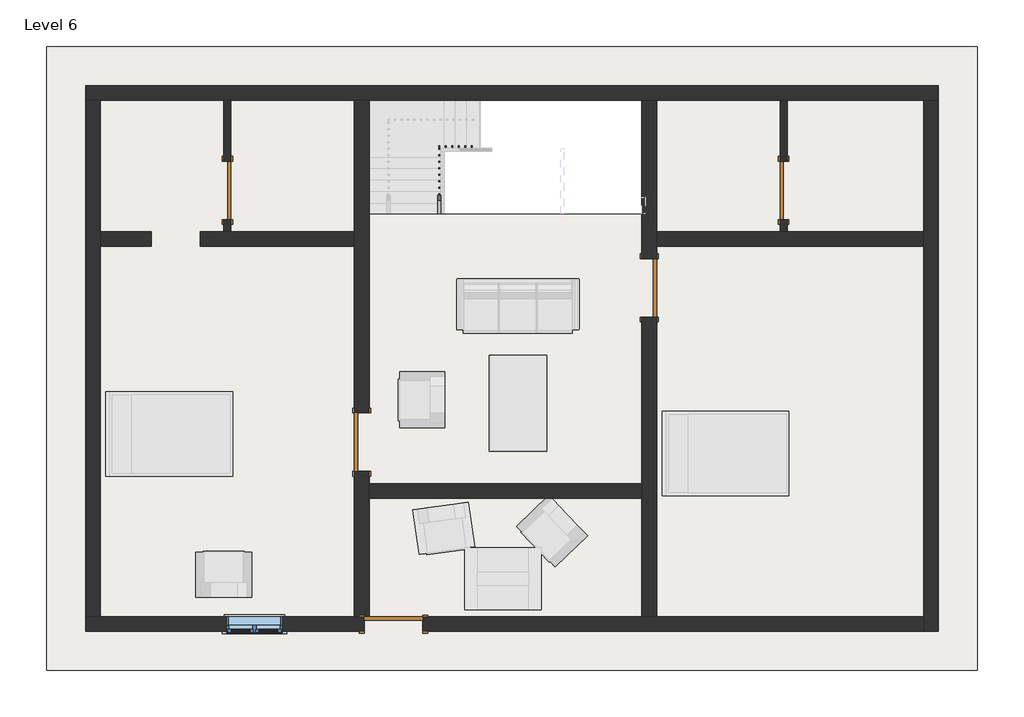
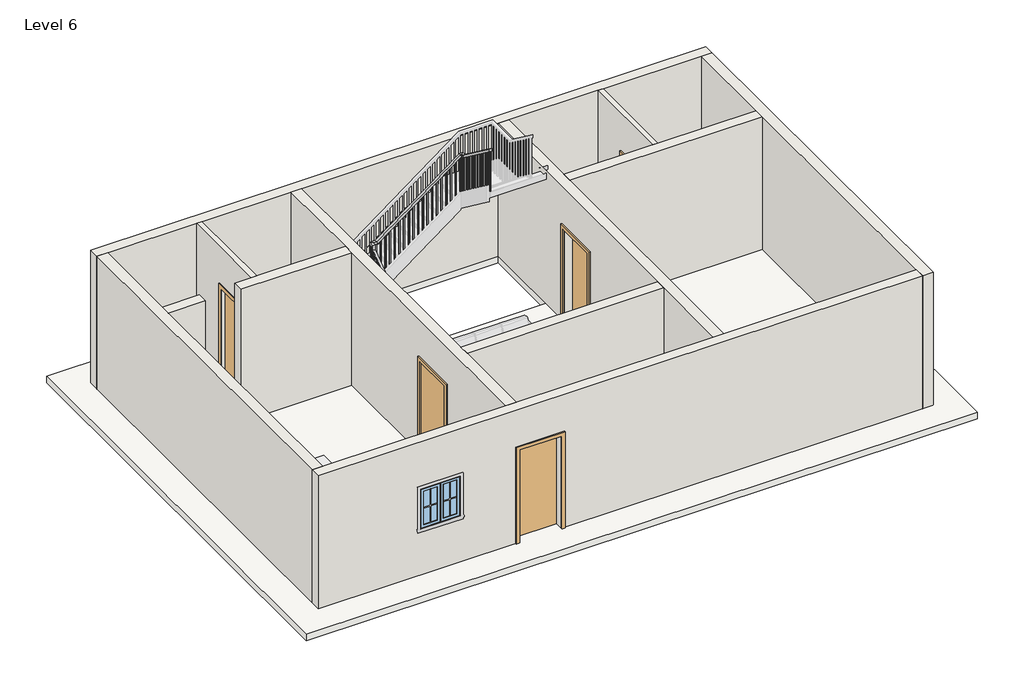
# One storey, part 1 of 2: 12 walls, 5 doors, 1 railing, 1 roof, 1 window.
"""IFC4 building model written with IfcOpenShell, lengths in millimetres."""

from ifc_helpers import new_model, si_unit, frame, origin, place, context, project, spatial, polyline, outline, extrude, faceted_brep, transform, mapped, element, save
from components import door_e5f9f3c4, door_a90ba1ad, door_305aa2a5, window_339605e1

model = new_model("IFC4")

# Units and contexts
model_context = context("Model", 3, world=origin())
ifc_project = project(units=[si_unit("LENGTHUNIT", "METRE", prefix="MILLI")], contexts=[model_context])

# Site, building, storey
site = spatial("IfcSite", under=ifc_project)
building = spatial("IfcBuilding", under=site)
storey = spatial("IfcBuildingStorey", under=building, Name="Level 6", Elevation=12801.6)

# Doors
placement = place(None, origin())
door_shape = door_e5f9f3c4(model_context)
element("IfcDoor", 1, ObjectType="Single-Flush : 36\" x 84\"", at=placement, inside=storey, context=model_context, shape_type="MappedRepresentation", body=[
    mapped(door_shape, transform((-5709.1546642, 5087.2167606, 12801.6), x_axis=(0.0, -1.0, 0.0), y_axis=(1.0, 0.0, 0.0), z_axis=(0.0, 0.0, 1.0))),
])
door_2_shape = door_a90ba1ad(model_context)
element("IfcDoor", 2, ObjectType="Single-Flush : 36\" x 84\"", at=placement, inside=storey, context=model_context, shape_type="MappedRepresentation", body=[
    mapped(door_2_shape, transform((-3607.3046642, 1150.2167606, 12801.6), x_axis=(0.0, -1.0, 0.0), y_axis=(1.0, 0.0, 0.0), z_axis=(0.0, 0.0, 1.0))),
])
element("IfcDoor", 3, ObjectType="Single-Flush : 36\" x 84\"", at=placement, inside=storey, context=model_context, shape_type="MappedRepresentation", body=[
    mapped(door_2_shape, transform((888.4953358, 3563.2167606, 12801.6), x_axis=(0.0, 1.0, 0.0), y_axis=(-1.0, 0.0, 0.0), z_axis=(0.0, 0.0, 1.0))),
])
element("IfcDoor", 4, ObjectType="Single-Flush : 36\" x 84\"", at=placement, inside=storey, context=model_context, shape_type="MappedRepresentation", body=[
    mapped(door_2_shape, transform((-3112.0046642, -1694.5832394, 12801.6), x_axis=(-1.0, 0.0, 0.0), y_axis=(0.0, -1.0, 0.0), z_axis=(0.0, 0.0, 1.0))),
])
door_3_shape = door_305aa2a5(model_context)
element("IfcDoor", 5, ObjectType="Single-Flush : 36\" x 84\"", at=placement, inside=storey, context=model_context, shape_type="MappedRepresentation", body=[
    mapped(door_3_shape, transform((2990.3453358, 5087.2167606, 12801.6), x_axis=(0.0, -1.0, 0.0), y_axis=(1.0, 0.0, 0.0), z_axis=(0.0, 0.0, 1.0))),
])

# Railing
element("IfcRailing", 6, ObjectType="Handrail - Rectangular", at=placement, inside=storey, context=model_context, shape_type="SolidModel", body=[
    faceted_brep([(-2419.4972892, 4718.9167606, 13848.5217391), (-2419.4972892, 4718.9167606, 13785.1634439), (-2368.6972892, 4718.9167606, 13785.1634439), (-2368.6972892, 4718.9167606, 13848.5217391), (-2419.4972892, 5670.3536537, 14557.6672495), (-2419.4972892, 5721.1536537, 14532.1723083), (-2368.6972892, 5721.1536537, 14532.1723083), (-2368.6972892, 5670.3536537, 14557.6672495), (-2419.4972892, 5670.3536537, 14664.4733611), (-2419.4972892, 5721.1536537, 14613.6733611), (-2368.6972892, 5721.1536537, 14613.6733611), (-2368.6972892, 5670.3536537, 14664.4733611), (-2419.4972892, 5797.3536537, 14664.4733611), (-2419.4972892, 5797.3536537, 14613.6733611), (-2368.6972892, 5746.5536537, 14613.6733611), (-2368.6972892, 5746.5536537, 14664.4733611), (-2292.4972892, 5797.3536537, 14664.4733611), (-2275.6482431, 5797.3536537, 14613.6733611), (-2275.6482431, 5746.5536537, 14613.6733611), (-2292.4972892, 5746.5536537, 14664.4733611), (-474.1369697, 5797.3536537, 16019.7729781), (-457.2879235, 5797.3536537, 15968.9729781), (-457.2879235, 5746.5536537, 15968.9729781), (-474.1369697, 5746.5536537, 16019.7729781), (-394.2046642, 5797.3536537, 16019.7729781), (-394.2046642, 5797.3536537, 15968.9729781), (-445.0046642, 5746.5536537, 15968.9729781), (-445.0046642, 5746.5536537, 16019.7729781), (-394.2046642, 5717.4213483, 16019.7729781), (-394.2046642, 5700.5723021, 15968.9729781), (-445.0046642, 5700.5723021, 15968.9729781), (-445.0046642, 5717.4213483, 16019.7729781), (-394.2046642, 4718.9167606, 16764.0), (-445.0046642, 4718.9167606, 16764.0), (-445.0046642, 4718.9167606, 16700.6417047), (-394.2046642, 4718.9167606, 16700.6417047)], [[[0, 1, 2, 3]], [[1, 0, 4, 5]], [[2, 1, 5, 6]], [[3, 2, 6, 7]], [[0, 3, 7, 4]], [[5, 4, 8, 9]], [[6, 5, 9, 10]], [[7, 6, 10, 11]], [[4, 7, 11, 8]], [[9, 8, 12, 13]], [[10, 9, 13, 14]], [[11, 10, 14, 15]], [[8, 11, 15, 12]], [[13, 12, 16, 17]], [[14, 13, 17, 18]], [[15, 14, 18, 19]], [[12, 15, 19, 16]], [[17, 16, 20, 21]], [[18, 17, 21, 22]], [[19, 18, 22, 23]], [[16, 19, 23, 20]], [[21, 20, 24, 25]], [[22, 21, 25, 26]], [[23, 22, 26, 27]], [[20, 23, 27, 24]], [[25, 24, 28, 29]], [[26, 25, 29, 30]], [[27, 26, 30, 31]], [[24, 27, 31, 28]], [[32, 33, 34, 35]], [[29, 28, 32, 35]], [[30, 29, 35, 34]], [[31, 30, 34, 33]], [[28, 31, 33, 32]]]),
    extrude(outline(polyline([(4746.4286537, 16680.1359459), (4765.4786537, 16665.9371882), (4765.4786537, 15717.0782609), (4746.4286537, 15717.0782609), (4746.4286537, 16680.1359459)])), frame((-429.1296642, 0.0, 0.0), z_axis=(1.0, 0.0, 0.0), x_axis=(0.0, 1.0, 0.0)), (0.0, 0.0, 1.0), 19.05),
    extrude(outline(polyline([(4848.0286537, 16604.4092378), (4867.0786537, 16590.2104801), (4867.0786537, 15717.0782609), (4848.0286537, 15717.0782609), (4848.0286537, 16604.4092378)])), frame((-429.1296642, 0.0, 0.0), z_axis=(1.0, 0.0, 0.0), x_axis=(0.0, 1.0, 0.0)), (0.0, 0.0, 1.0), 19.05),
    extrude(outline(polyline([(4949.6286537, 16528.6825298), (4968.6786537, 16514.483772), (4968.6786537, 15584.5565217), (4949.6286537, 15584.5565217), (4949.6286537, 16528.6825298)])), frame((-429.1296642, 0.0, 0.0), z_axis=(1.0, 0.0, 0.0), x_axis=(0.0, 1.0, 0.0)), (0.0, 0.0, 1.0), 19.05),
    extrude(outline(polyline([(5051.2286537, 16452.9558217), (5070.2786537, 16438.7570639), (5070.2786537, 15584.5565217), (5051.2286537, 15584.5565217), (5051.2286537, 16452.9558217)])), frame((-429.1296642, 0.0, 0.0), z_axis=(1.0, 0.0, 0.0), x_axis=(0.0, 1.0, 0.0)), (0.0, 0.0, 1.0), 19.05),
    extrude(outline(polyline([(5152.8286537, 16377.2291136), (5171.8786537, 16363.0303559), (5171.8786537, 15452.0347826), (5152.8286537, 15452.0347826), (5152.8286537, 16377.2291136)])), frame((-429.1296642, 0.0, 0.0), z_axis=(1.0, 0.0, 0.0), x_axis=(0.0, 1.0, 0.0)), (0.0, 0.0, 1.0), 19.05),
    extrude(outline(polyline([(5254.4286537, 16301.5024055), (5273.4786537, 16287.3036478), (5273.4786537, 15319.5130435), (5254.4286537, 15319.5130435), (5254.4286537, 16301.5024055)])), frame((-429.1296642, 0.0, 0.0), z_axis=(1.0, 0.0, 0.0), x_axis=(0.0, 1.0, 0.0)), (0.0, 0.0, 1.0), 19.05),
    extrude(outline(polyline([(5356.0286537, 16225.7756975), (5375.0786537, 16211.5769397), (5375.0786537, 15319.5130435), (5356.0286537, 15319.5130435), (5356.0286537, 16225.7756975)])), frame((-429.1296642, 0.0, 0.0), z_axis=(1.0, 0.0, 0.0), x_axis=(0.0, 1.0, 0.0)), (0.0, 0.0, 1.0), 19.05),
    extrude(outline(polyline([(5457.6286537, 16150.0489894), (5476.6786537, 16135.8502316), (5476.6786537, 15186.9913043), (5457.6286537, 15186.9913043), (5457.6286537, 16150.0489894)])), frame((-429.1296642, 0.0, 0.0), z_axis=(1.0, 0.0, 0.0), x_axis=(0.0, 1.0, 0.0)), (0.0, 0.0, 1.0), 19.05),
    extrude(outline(polyline([(5559.2286537, 16074.3222813), (5578.2786537, 16060.1235236), (5578.2786537, 15186.9913043), (5559.2286537, 15186.9913043), (5559.2286537, 16074.3222813)])), frame((-429.1296642, 0.0, 0.0), z_axis=(1.0, 0.0, 0.0), x_axis=(0.0, 1.0, 0.0)), (0.0, 0.0, 1.0), 19.05),
    extrude(outline(polyline([(5660.8286537, 15998.5955732), (5679.8786537, 15984.3968155), (5679.8786537, 15054.4695652), (5660.8286537, 15054.4695652), (5660.8286537, 15998.5955732)])), frame((-429.1296642, 0.0, 0.0), z_axis=(1.0, 0.0, 0.0), x_axis=(0.0, 1.0, 0.0)), (0.0, 0.0, 1.0), 19.05),
    extrude(outline(polyline([(-473.2222892, 5762.4286537), (-473.2222892, 5781.4786537), (-454.1722892, 5781.4786537), (-454.1722892, 5762.4286537), (-473.2222892, 5762.4286537)])), frame((0.0, 0.0, 15054.4695652), z_axis=(0.0, 0.0, 1.0), x_axis=(1.0, 0.0, 0.0)), (0.0, 0.0, 1.0), 914.5034129),
    extrude(outline(polyline([(15895.5684819, -555.7722892), (15881.3697242, -574.8222892), (14921.9478261, -574.8222892), (14921.9478261, -555.7722892), (15895.5684819, -555.7722892)])), frame((0.0, 5762.4286537, 0.0), z_axis=(0.0, 1.0, 0.0), x_axis=(0.0, 0.0, 1.0)), (0.0, 0.0, 1.0), 19.05),
    extrude(outline(polyline([(15819.8417739, -657.3722892), (15805.6430161, -676.4222892), (14921.9478261, -676.4222892), (14921.9478261, -657.3722892), (15819.8417739, -657.3722892)])), frame((0.0, 5762.4286537, 0.0), z_axis=(0.0, 1.0, 0.0), x_axis=(0.0, 0.0, 1.0)), (0.0, 0.0, 1.0), 19.05),
    extrude(outline(polyline([(15744.1150658, -758.9722892), (15729.916308, -778.0222892), (14789.426087, -778.0222892), (14789.426087, -758.9722892), (15744.1150658, -758.9722892)])), frame((0.0, 5762.4286537, 0.0), z_axis=(0.0, 1.0, 0.0), x_axis=(0.0, 0.0, 1.0)), (0.0, 0.0, 1.0), 19.05),
    extrude(outline(polyline([(15668.3883577, -860.5722892), (15654.1896, -879.6222892), (14789.426087, -879.6222892), (14789.426087, -860.5722892), (15668.3883577, -860.5722892)])), frame((0.0, 5762.4286537, 0.0), z_axis=(0.0, 1.0, 0.0), x_axis=(0.0, 0.0, 1.0)), (0.0, 0.0, 1.0), 19.05),
    extrude(outline(polyline([(15592.6616496, -962.1722892), (15578.4628919, -981.2222892), (14656.9043478, -981.2222892), (14656.9043478, -962.1722892), (15592.6616496, -962.1722892)])), frame((0.0, 5762.4286537, 0.0), z_axis=(0.0, 1.0, 0.0), x_axis=(0.0, 0.0, 1.0)), (0.0, 0.0, 1.0), 19.05),
    extrude(outline(polyline([(15516.9349416, -1063.7722892), (15502.7361838, -1082.8222892), (14656.9043478, -1082.8222892), (14656.9043478, -1063.7722892), (15516.9349416, -1063.7722892)])), frame((0.0, 5762.4286537, 0.0), z_axis=(0.0, 1.0, 0.0), x_axis=(0.0, 0.0, 1.0)), (0.0, 0.0, 1.0), 19.05),
    extrude(outline(polyline([(15441.2082335, -1165.3722892), (15427.0094757, -1184.4222892), (14524.3826087, -1184.4222892), (14524.3826087, -1165.3722892), (15441.2082335, -1165.3722892)])), frame((0.0, 5762.4286537, 0.0), z_axis=(0.0, 1.0, 0.0), x_axis=(0.0, 0.0, 1.0)), (0.0, 0.0, 1.0), 19.05),
    extrude(outline(polyline([(15365.4815254, -1266.9722892), (15351.2827677, -1286.0222892), (14391.8608696, -1286.0222892), (14391.8608696, -1266.9722892), (15365.4815254, -1266.9722892)])), frame((0.0, 5762.4286537, 0.0), z_axis=(0.0, 1.0, 0.0), x_axis=(0.0, 0.0, 1.0)), (0.0, 0.0, 1.0), 19.05),
    extrude(outline(polyline([(15289.7548173, -1368.5722892), (15275.5560596, -1387.6222892), (14391.8608696, -1387.6222892), (14391.8608696, -1368.5722892), (15289.7548173, -1368.5722892)])), frame((0.0, 5762.4286537, 0.0), z_axis=(0.0, 1.0, 0.0), x_axis=(0.0, 0.0, 1.0)), (0.0, 0.0, 1.0), 19.05),
    extrude(outline(polyline([(15214.0281093, -1470.1722892), (15199.8293515, -1489.2222892), (14259.3391304, -1489.2222892), (14259.3391304, -1470.1722892), (15214.0281093, -1470.1722892)])), frame((0.0, 5762.4286537, 0.0), z_axis=(0.0, 1.0, 0.0), x_axis=(0.0, 0.0, 1.0)), (0.0, 0.0, 1.0), 19.05),
    extrude(outline(polyline([(15138.3014012, -1571.7722892), (15124.1026434, -1590.8222892), (14259.3391304, -1590.8222892), (14259.3391304, -1571.7722892), (15138.3014012, -1571.7722892)])), frame((0.0, 5762.4286537, 0.0), z_axis=(0.0, 1.0, 0.0), x_axis=(0.0, 0.0, 1.0)), (0.0, 0.0, 1.0), 19.05),
    extrude(outline(polyline([(15062.5746931, -1673.3722892), (15048.3759354, -1692.4222892), (14126.8173913, -1692.4222892), (14126.8173913, -1673.3722892), (15062.5746931, -1673.3722892)])), frame((0.0, 5762.4286537, 0.0), z_axis=(0.0, 1.0, 0.0), x_axis=(0.0, 0.0, 1.0)), (0.0, 0.0, 1.0), 19.05),
    extrude(outline(polyline([(14986.847985, -1774.9722892), (14972.6492273, -1794.0222892), (14126.8173913, -1794.0222892), (14126.8173913, -1774.9722892), (14986.847985, -1774.9722892)])), frame((0.0, 5762.4286537, 0.0), z_axis=(0.0, 1.0, 0.0), x_axis=(0.0, 0.0, 1.0)), (0.0, 0.0, 1.0), 19.05),
    extrude(outline(polyline([(14911.121277, -1876.5722892), (14896.9225192, -1895.6222892), (13994.2956522, -1895.6222892), (13994.2956522, -1876.5722892), (14911.121277, -1876.5722892)])), frame((0.0, 5762.4286537, 0.0), z_axis=(0.0, 1.0, 0.0), x_axis=(0.0, 0.0, 1.0)), (0.0, 0.0, 1.0), 19.05),
    extrude(outline(polyline([(14835.3945689, -1978.1722892), (14821.1958111, -1997.2222892), (13861.773913, -1997.2222892), (13861.773913, -1978.1722892), (14835.3945689, -1978.1722892)])), frame((0.0, 5762.4286537, 0.0), z_axis=(0.0, 1.0, 0.0), x_axis=(0.0, 0.0, 1.0)), (0.0, 0.0, 1.0), 19.05),
    extrude(outline(polyline([(14759.6678608, -2079.7722892), (14745.4691031, -2098.8222892), (13861.773913, -2098.8222892), (13861.773913, -2079.7722892), (14759.6678608, -2079.7722892)])), frame((0.0, 5762.4286537, 0.0), z_axis=(0.0, 1.0, 0.0), x_axis=(0.0, 0.0, 1.0)), (0.0, 0.0, 1.0), 19.05),
    extrude(outline(polyline([(14683.9411527, -2181.3722892), (14669.742395, -2200.4222892), (13729.2521739, -2200.4222892), (13729.2521739, -2181.3722892), (14683.9411527, -2181.3722892)])), frame((0.0, 5762.4286537, 0.0), z_axis=(0.0, 1.0, 0.0), x_axis=(0.0, 0.0, 1.0)), (0.0, 0.0, 1.0), 19.05),
    extrude(outline(polyline([(14608.2144447, -2282.9722892), (14594.0156869, -2302.0222892), (13729.2521739, -2302.0222892), (13729.2521739, -2282.9722892), (14608.2144447, -2282.9722892)])), frame((0.0, 5762.4286537, 0.0), z_axis=(0.0, 1.0, 0.0), x_axis=(0.0, 0.0, 1.0)), (0.0, 0.0, 1.0), 19.05),
    extrude(outline(polyline([(-2384.5722892, 5725.3917606), (-2403.6222892, 5725.3917606), (-2403.6222892, 5744.4417606), (-2384.5722892, 5744.4417606), (-2384.5722892, 5725.3917606)])), frame((0.0, 0.0, 13596.7304348), z_axis=(0.0, 0.0, 1.0), x_axis=(1.0, 0.0, 0.0)), (0.0, 0.0, 1.0), 1016.9429263),
    extrude(outline(polyline([(5623.7917606, 14459.6044377), (5642.8417606, 14473.8031954), (5642.8417606, 13596.7304348), (5623.7917606, 13596.7304348), (5623.7917606, 14459.6044377)])), frame((-2403.6222892, 0.0, 0.0), z_axis=(1.0, 0.0, 0.0), x_axis=(0.0, 1.0, 0.0)), (0.0, 0.0, 1.0), 19.05),
    extrude(outline(polyline([(5522.1917606, 14383.8777296), (5541.2417606, 14398.0764873), (5541.2417606, 13464.2086957), (5522.1917606, 13464.2086957), (5522.1917606, 14383.8777296)])), frame((-2403.6222892, 0.0, 0.0), z_axis=(1.0, 0.0, 0.0), x_axis=(0.0, 1.0, 0.0)), (0.0, 0.0, 1.0), 19.05),
    extrude(outline(polyline([(5420.5917606, 14308.1510215), (5439.6417606, 14322.3497793), (5439.6417606, 13464.2086957), (5420.5917606, 13464.2086957), (5420.5917606, 14308.1510215)])), frame((-2403.6222892, 0.0, 0.0), z_axis=(1.0, 0.0, 0.0), x_axis=(0.0, 1.0, 0.0)), (0.0, 0.0, 1.0), 19.05),
    extrude(outline(polyline([(5318.9917606, 14232.4243134), (5338.0417606, 14246.6230712), (5338.0417606, 13331.6869565), (5318.9917606, 13331.6869565), (5318.9917606, 14232.4243134)])), frame((-2403.6222892, 0.0, 0.0), z_axis=(1.0, 0.0, 0.0), x_axis=(0.0, 1.0, 0.0)), (0.0, 0.0, 1.0), 19.05),
    extrude(outline(polyline([(5217.3917606, 14156.6976054), (5236.4417606, 14170.8963631), (5236.4417606, 13199.1652174), (5217.3917606, 13199.1652174), (5217.3917606, 14156.6976054)])), frame((-2403.6222892, 0.0, 0.0), z_axis=(1.0, 0.0, 0.0), x_axis=(0.0, 1.0, 0.0)), (0.0, 0.0, 1.0), 19.05),
    extrude(outline(polyline([(5115.7917606, 14080.9708973), (5134.8417606, 14095.169655), (5134.8417606, 13199.1652174), (5115.7917606, 13199.1652174), (5115.7917606, 14080.9708973)])), frame((-2403.6222892, 0.0, 0.0), z_axis=(1.0, 0.0, 0.0), x_axis=(0.0, 1.0, 0.0)), (0.0, 0.0, 1.0), 19.05),
    extrude(outline(polyline([(5014.1917606, 14005.2441892), (5033.2417606, 14019.442947), (5033.2417606, 13066.6434783), (5014.1917606, 13066.6434783), (5014.1917606, 14005.2441892)])), frame((-2403.6222892, 0.0, 0.0), z_axis=(1.0, 0.0, 0.0), x_axis=(0.0, 1.0, 0.0)), (0.0, 0.0, 1.0), 19.05),
    extrude(outline(polyline([(4912.5917606, 13929.5174811), (4931.6417606, 13943.7162389), (4931.6417606, 13066.6434783), (4912.5917606, 13066.6434783), (4912.5917606, 13929.5174811)])), frame((-2403.6222892, 0.0, 0.0), z_axis=(1.0, 0.0, 0.0), x_axis=(0.0, 1.0, 0.0)), (0.0, 0.0, 1.0), 19.05),
    extrude(outline(polyline([(4810.9917606, 13853.7907731), (4830.0417606, 13867.9895308), (4830.0417606, 12934.1217391), (4810.9917606, 12934.1217391), (4810.9917606, 13853.7907731)])), frame((-2403.6222892, 0.0, 0.0), z_axis=(1.0, 0.0, 0.0), x_axis=(0.0, 1.0, 0.0)), (0.0, 0.0, 1.0), 19.05),
    extrude(outline(polyline([(-429.1296642, 5762.4286537), (-429.1296642, 5781.4786537), (-410.0796642, 5781.4786537), (-410.0796642, 5762.4286537), (-429.1296642, 5762.4286537)])), frame((0.0, 0.0, 15054.4695652), z_axis=(0.0, 0.0, 1.0), x_axis=(1.0, 0.0, 0.0)), (0.0, 0.0, 1.0), 914.5034129),
    extrude(outline(polyline([(-2384.5722892, 5762.4286537), (-2403.6222892, 5762.4286537), (-2403.6222892, 5781.4786537), (-2384.5722892, 5781.4786537), (-2384.5722892, 5762.4286537)])), frame((0.0, 0.0, 13596.7304348), z_axis=(0.0, 0.0, 1.0), x_axis=(1.0, 0.0, 0.0)), (0.0, 0.0, 1.0), 1016.9429263),
    extrude(outline(polyline([(4718.9167606, 16700.6417047), (4737.9667606, 16686.442947), (4737.9667606, 15717.0782609), (4718.9167606, 15717.0782609), (4718.9167606, 16700.6417047)])), frame((-429.1296642, 0.0, 0.0), z_axis=(1.0, 0.0, 0.0), x_axis=(0.0, 1.0, 0.0)), (0.0, 0.0, 1.0), 19.05),
    extrude(outline(polyline([(4718.9167606, 13785.1634439), (4737.9667606, 13799.3622016), (4737.9667606, 12934.1217391), (4718.9167606, 12934.1217391), (4718.9167606, 13785.1634439)])), frame((-2403.6222892, 0.0, 0.0), z_axis=(1.0, 0.0, 0.0), x_axis=(0.0, 1.0, 0.0)), (0.0, 0.0, 1.0), 19.05),
])

# Roof
element("IfcRoof", 7, ObjectType="Generic - 12\"", at=placement, inside=storey, context=model_context, shape_type="SweptSolid", body=[
    extrude(outline(polyline([(6019.2953358, 7335.1167606), (6019.2953358, -2418.4832394), (-8534.9046642, -2418.4832394), (-8534.9046642, 7335.1167606), (6019.2953358, 7335.1167606)]), holes=[polyline([(774.1953358, 6496.9167606), (-3493.0046642, 6496.9167606), (-3493.0046642, 4718.9167606), (774.1953358, 4718.9167606), (774.1953358, 6496.9167606)])]), frame((0.0, 0.0, 12649.2), z_axis=(0.0, 0.0, 1.0), x_axis=(1.0, 0.0, 0.0)), (0.0, 0.0, 1.0), 152.4),
])

# Walls
element("IfcWall", 8, ObjectType="WALL4.5\"", at=placement, inside=storey, context=model_context, shape_type="SweptSolid", body=[
    extrude(outline(polyline([(4630.0167606, 14935.2), (4630.0167606, 12801.6), (4439.5167606, 12801.6), (4439.5167606, 15849.6), (6496.9167606, 15849.6), (6496.9167606, 12801.6), (5544.4167606, 12801.6), (5544.4167606, 14935.2), (4630.0167606, 14935.2)])), frame((-5766.3046642, 0.0, 0.0), z_axis=(1.0, 0.0, 0.0), x_axis=(0.0, 1.0, 0.0)), (0.0, 0.0, 1.0), 114.3),
])
element("IfcWall", 9, ObjectType="WALL4.5\"", at=placement, inside=storey, context=model_context, shape_type="SweptSolid", body=[
    extrude(outline(polyline([(4630.0167606, 14935.2), (4630.0167606, 12801.6), (4439.5167606, 12801.6), (4439.5167606, 15849.6), (6496.9167606, 15849.6), (6496.9167606, 12801.6), (5544.4167606, 12801.6), (5544.4167606, 14935.2), (4630.0167606, 14935.2)])), frame((2933.1953358, 0.0, 0.0), z_axis=(1.0, 0.0, 0.0), x_axis=(0.0, 1.0, 0.0)), (0.0, 0.0, 1.0), 114.3),
])
element("IfcWall", 10, ObjectType="WALL9\"", at=placement, inside=storey, context=model_context, shape_type="Brep", body=[
    faceted_brep([(-7925.3046642, 6496.9167606, 12801.6), (-7696.7046642, 6496.9167606, 12801.6), (-5766.3046642, 6496.9167606, 12801.6), (-5652.0046642, 6496.9167606, 12801.6), (-3721.6046642, 6496.9167606, 12801.6), (-3493.0046642, 6496.9167606, 12801.6), (774.1953358, 6496.9167606, 12801.6), (1002.7953358, 6496.9167606, 12801.6), (2933.1953358, 6496.9167606, 12801.6), (3047.4953358, 6496.9167606, 12801.6), (5181.0953358, 6496.9167606, 12801.6), (5409.6953358, 6496.9167606, 12801.6), (5409.6953358, 6496.9167606, 15849.6), (5181.0953358, 6496.9167606, 15849.6), (3047.4953358, 6496.9167606, 15849.6), (2933.1953358, 6496.9167606, 15849.6), (1002.7953358, 6496.9167606, 15849.6), (774.1953358, 6496.9167606, 15849.6), (-3493.0046642, 6496.9167606, 15849.6), (-3721.6046642, 6496.9167606, 15849.6), (-5652.0046642, 6496.9167606, 15849.6), (-5766.3046642, 6496.9167606, 15849.6), (-7696.7046642, 6496.9167606, 15849.6), (-7925.3046642, 6496.9167606, 15849.6), (-7925.3046642, 6725.5167606, 12801.6), (-7925.3046642, 6725.5167606, 15849.6), (5409.6953358, 6725.5167606, 15849.6), (5409.6953358, 6725.5167606, 12801.6)], [[[0, 1, 2, 3, 4, 5, 6, 7, 8, 9, 10, 11, 12, 13, 14, 15, 16, 17, 18, 19, 20, 21, 22, 23]], [[24, 25, 26, 27]], [[11, 10, 9, 8, 7, 6, 5, 4, 3, 2, 1, 0, 24, 27]], [[12, 11, 27, 26]], [[0, 23, 25, 24]], [[23, 22, 21, 20, 19, 18, 17, 16, 15, 14, 13, 12, 26, 25]]]),
])
element("IfcWall", 11, ObjectType="WALL9\"", at=placement, inside=storey, context=model_context, shape_type="Brep", body=[
    faceted_brep([(5181.0953358, 6496.9167606, 12801.6), (5181.0953358, 4439.5167606, 12801.6), (5181.0953358, 4210.9167606, 12801.6), (5181.0953358, -1580.2832394, 12801.6), (5181.0953358, -1808.8832394, 12801.6), (5181.0953358, -1808.8832394, 15849.6), (5181.0953358, -1580.2832394, 15849.6), (5181.0953358, 4210.9167606, 15849.6), (5181.0953358, 4439.5167606, 15849.6), (5181.0953358, 6496.9167606, 15849.6), (5409.6953358, 6496.9167606, 12801.6), (5409.6953358, 6496.9167606, 15849.6), (5409.6953358, -1808.8832394, 15849.6), (5409.6953358, -1808.8832394, 12801.6)], [[[0, 1, 2, 3, 4, 5, 6, 7, 8, 9]], [[10, 11, 12, 13]], [[4, 3, 2, 1, 0, 10, 13]], [[0, 9, 11, 10]], [[5, 4, 13, 12]], [[9, 8, 7, 6, 5, 12, 11]]]),
])
element("IfcWall", 12, ObjectType="WALL9\"", at=placement, inside=storey, context=model_context, shape_type="Brep", body=[
    faceted_brep([(-3569.2046642, -1580.2832394, 14935.2), (-3569.2046642, -1580.2832394, 12801.6), (-3721.6046642, -1580.2832394, 12801.6), (-7696.7046642, -1580.2832394, 12801.6), (-7925.3046642, -1580.2832394, 12801.6), (-7925.3046642, -1580.2832394, 15849.6), (-7696.7046642, -1580.2832394, 15849.6), (-3721.6046642, -1580.2832394, 15849.6), (-3493.0046642, -1580.2832394, 15849.6), (774.1953358, -1580.2832394, 15849.6), (1002.7953358, -1580.2832394, 15849.6), (5181.0953358, -1580.2832394, 15849.6), (5181.0953358, -1580.2832394, 12801.6), (1002.7953358, -1580.2832394, 12801.6), (774.1953358, -1580.2832394, 12801.6), (-2654.8046642, -1580.2832394, 12801.6), (-2654.8046642, -1580.2832394, 14935.2), (-5715.5046642, -1580.2832394, 14783.1434313), (-5715.5046642, -1580.2832394, 13868.7434313), (-4851.9046642, -1580.2832394, 13868.7434313), (-4851.9046642, -1580.2832394, 14783.1434313), (-7925.3046642, -1808.8832394, 12801.6), (-3569.2046642, -1808.8832394, 12801.6), (-3569.2046642, -1808.8832394, 14935.2), (-2654.8046642, -1808.8832394, 14935.2), (-2654.8046642, -1808.8832394, 12801.6), (5181.0953358, -1808.8832394, 12801.6), (5181.0953358, -1808.8832394, 15849.6), (-7925.3046642, -1808.8832394, 15849.6), (-5715.5046642, -1808.8832394, 14783.1434313), (-4851.9046642, -1808.8832394, 14783.1434313), (-4851.9046642, -1808.8832394, 13868.7434313), (-5715.5046642, -1808.8832394, 13868.7434313)], [[[0, 1, 2, 3, 4, 5, 6, 7, 8, 9, 10, 11, 12, 13, 14, 15, 16], [17, 18, 19, 20]], [[21, 22, 23, 24, 25, 26, 27, 28], [29, 30, 31, 32]], [[4, 3, 2, 1, 22, 21]], [[15, 14, 13, 12, 26, 25]], [[12, 11, 27, 26]], [[5, 4, 21, 28]], [[23, 22, 1, 0]], [[24, 23, 0, 16]], [[25, 24, 16, 15]], [[11, 10, 9, 8, 7, 6, 5, 28, 27]], [[18, 17, 29, 32]], [[19, 18, 32, 31]], [[20, 19, 31, 30]], [[17, 20, 30, 29]]]),
])
element("IfcWall", 13, ObjectType="WALL9\"", at=placement, inside=storey, context=model_context, shape_type="Brep", body=[
    faceted_brep([(-7696.7046642, -1580.2832394, 12801.6), (-7696.7046642, 4210.9167606, 12801.6), (-7696.7046642, 4439.5167606, 12801.6), (-7696.7046642, 6496.9167606, 12801.6), (-7696.7046642, 6496.9167606, 15849.6), (-7696.7046642, 4439.5167606, 15849.6), (-7696.7046642, 4210.9167606, 15849.6), (-7696.7046642, -1580.2832394, 15849.6), (-7925.3046642, -1580.2832394, 12801.6), (-7925.3046642, -1580.2832394, 15849.6), (-7925.3046642, 6496.9167606, 15849.6), (-7925.3046642, 6496.9167606, 12801.6)], [[[0, 1, 2, 3, 4, 5, 6, 7]], [[8, 9, 10, 11]], [[3, 2, 1, 0, 8, 11]], [[4, 3, 11, 10]], [[0, 7, 9, 8]], [[7, 6, 5, 4, 10, 9]]]),
])
element("IfcWall", 14, ObjectType="WALL9\"", at=placement, inside=storey, context=model_context, shape_type="Brep", body=[
    faceted_brep([(-3721.6046642, 693.0167606, 14935.2), (-3721.6046642, 693.0167606, 12801.6), (-3721.6046642, -1580.2832394, 12801.6), (-3721.6046642, -1580.2832394, 15849.6), (-3721.6046642, 4210.9167606, 15849.6), (-3721.6046642, 4439.5167606, 15849.6), (-3721.6046642, 6496.9167606, 15849.6), (-3721.6046642, 6496.9167606, 12801.6), (-3721.6046642, 4439.5167606, 12801.6), (-3721.6046642, 4210.9167606, 12801.6), (-3721.6046642, 1607.4167606, 12801.6), (-3721.6046642, 1607.4167606, 14935.2), (-3493.0046642, -1580.2832394, 12801.6), (-3493.0046642, 273.9167606, 12801.6), (-3493.0046642, 502.5167606, 12801.6), (-3493.0046642, 693.0167606, 12801.6), (-3493.0046642, 693.0167606, 14935.2), (-3493.0046642, 1607.4167606, 14935.2), (-3493.0046642, 1607.4167606, 12801.6), (-3493.0046642, 6496.9167606, 12801.6), (-3493.0046642, 6496.9167606, 15849.6), (-3493.0046642, 4718.9167606, 15849.6), (-3493.0046642, 502.5167606, 15849.6), (-3493.0046642, 273.9167606, 15849.6), (-3493.0046642, -1580.2832394, 15849.6), (-3569.2046642, -1580.2832394, 12801.6)], [[[0, 1, 2, 3, 4, 5, 6, 7, 8, 9, 10, 11]], [[12, 13, 14, 15, 16, 17, 18, 19, 20, 21, 22, 23, 24]], [[2, 1, 15, 14, 13, 12, 25]], [[10, 9, 8, 7, 19, 18]], [[7, 6, 20, 19]], [[3, 2, 25, 12, 24]], [[16, 15, 1, 0]], [[17, 16, 0, 11]], [[18, 17, 11, 10]], [[6, 5, 4, 3, 24, 23, 22, 21, 20]]]),
])
element("IfcWall", 15, ObjectType="WALL9\"", at=placement, inside=storey, context=model_context, shape_type="Brep", body=[
    faceted_brep([(774.1953358, 6496.9167606, 12801.6), (774.1953358, 4020.4167606, 12801.6), (774.1953358, 4020.4167606, 14935.2), (774.1953358, 3106.0167606, 14935.2), (774.1953358, 3106.0167606, 12801.6), (774.1953358, 502.5167606, 12801.6), (774.1953358, 273.9167606, 12801.6), (774.1953358, -1580.2832394, 12801.6), (774.1953358, -1580.2832394, 15849.6), (774.1953358, 273.9167606, 15849.6), (774.1953358, 502.5167606, 15849.6), (774.1953358, 4718.9167606, 15849.6), (774.1953358, 6496.9167606, 15849.6), (1002.7953358, 4020.4167606, 14935.2), (1002.7953358, 4020.4167606, 12801.6), (1002.7953358, 4210.9167606, 12801.6), (1002.7953358, 4439.5167606, 12801.6), (1002.7953358, 6496.9167606, 12801.6), (1002.7953358, 6496.9167606, 15849.6), (1002.7953358, 4439.5167606, 15849.6), (1002.7953358, 4210.9167606, 15849.6), (1002.7953358, -1580.2832394, 15849.6), (1002.7953358, -1580.2832394, 12801.6), (1002.7953358, 3106.0167606, 12801.6), (1002.7953358, 3106.0167606, 14935.2)], [[[0, 1, 2, 3, 4, 5, 6, 7, 8, 9, 10, 11, 12]], [[13, 14, 15, 16, 17, 18, 19, 20, 21, 22, 23, 24]], [[23, 22, 7, 6, 5, 4]], [[17, 16, 15, 14, 1, 0]], [[0, 12, 18, 17]], [[8, 7, 22, 21]], [[2, 1, 14, 13]], [[3, 2, 13, 24]], [[4, 3, 24, 23]], [[12, 11, 10, 9, 8, 21, 20, 19, 18]]]),
])
element("IfcWall", 16, ObjectType="WALL9\"", at=placement, inside=storey, context=model_context, shape_type="SweptSolid", body=[
    extrude(outline(polyline([(774.1953358, 273.9167606), (-3493.0046642, 273.9167606), (-3493.0046642, 502.5167606), (774.1953358, 502.5167606), (774.1953358, 273.9167606)])), frame((0.0, 0.0, 12801.6), z_axis=(0.0, 0.0, 1.0), x_axis=(1.0, 0.0, 0.0)), (0.0, 0.0, 1.0), 3048.0),
])
element("IfcWall", 17, ObjectType="WALL9\"", at=placement, inside=storey, context=model_context, shape_type="SweptSolid", body=[
    extrude(outline(polyline([(-6895.4507894, 4210.9167606), (-7696.7046642, 4210.9167606), (-7696.7046642, 4439.5167606), (-6895.4507894, 4439.5167606), (-6895.4507894, 4210.9167606)])), frame((0.0, 0.0, 12801.6), z_axis=(0.0, 0.0, 1.0), x_axis=(1.0, 0.0, 0.0)), (0.0, 0.0, 1.0), 3048.0),
])
element("IfcWall", 18, ObjectType="WALL9\"", at=placement, inside=storey, context=model_context, shape_type="Brep", body=[
    faceted_brep([(-3721.6046642, 4439.5167606, 12801.6), (-5652.0046642, 4439.5167606, 12801.6), (-5766.3046642, 4439.5167606, 12801.6), (-6131.0963491, 4439.5167606, 12801.6), (-6131.0963491, 4439.5167606, 15849.6), (-5766.3046642, 4439.5167606, 15849.6), (-5652.0046642, 4439.5167606, 15849.6), (-3721.6046642, 4439.5167606, 15849.6), (-3721.6046642, 4210.9167606, 12801.6), (-3721.6046642, 4210.9167606, 15849.6), (-6131.0963491, 4210.9167606, 15849.6), (-6131.0963491, 4210.9167606, 12801.6)], [[[0, 1, 2, 3, 4, 5, 6, 7]], [[8, 9, 10, 11]], [[3, 2, 1, 0, 8, 11]], [[4, 3, 11, 10]], [[0, 7, 9, 8]], [[7, 6, 5, 4, 10, 9]]]),
])
element("IfcWall", 19, ObjectType="WALL9\"", at=placement, inside=storey, context=model_context, shape_type="Brep", body=[
    faceted_brep([(1002.7953358, 4210.9167606, 12801.6), (5181.0953358, 4210.9167606, 12801.6), (5181.0953358, 4210.9167606, 15849.6), (1002.7953358, 4210.9167606, 15849.6), (1002.7953358, 4439.5167606, 12801.6), (1002.7953358, 4439.5167606, 15849.6), (2933.1953358, 4439.5167606, 15849.6), (3047.4953358, 4439.5167606, 15849.6), (5181.0953358, 4439.5167606, 15849.6), (5181.0953358, 4439.5167606, 12801.6), (3047.4953358, 4439.5167606, 12801.6), (2933.1953358, 4439.5167606, 12801.6)], [[[0, 1, 2, 3]], [[4, 5, 6, 7, 8, 9, 10, 11]], [[1, 0, 4, 11, 10, 9]], [[2, 1, 9, 8]], [[0, 3, 5, 4]], [[3, 2, 8, 7, 6, 5]]]),
])

# Window
window_shape = window_339605e1(model_context)
element("IfcWindow", 20, ObjectType="Window-Casement-Double : 34\" x 36\"", at=placement, inside=storey, context=model_context, shape_type="MappedRepresentation", body=[
    mapped(window_shape, transform((-5283.7046642, -1694.5832394, 12954.3434313), x_axis=(-1.0, 0.0, 0.0), y_axis=(0.0, -1.0, 0.0), z_axis=(0.0, 0.0, 1.0))),
])

save(model, "model.ifc")

# Revit data of these elements
# Type "Single-Flush : 36\" x 84\""
#   Type Mark = "1"
#   Construction Type Id = "MDOOR"
#   Assembly Code = "C1020"
#   Analytic Construction = "Metal"
#   Thickness = 0' - 2"
#   Heat Transfer Coefficient (U) = 0.651978 BTU/(h·ft²·°F)
#   Height = 7' - 0"
#   Trim Projection Ext = 0' - 1"
#   Trim Projection Int = 0' - 1"
#   Trim Width = 0' - 3"
#   Width = 3' - 0"
#   Define Thermal Properties by = 1
#   Define Thermal Properties by = 1
#   Door Material = Door - Panel
#   Frame Material = Door - Frame
#   Visual Light Transmittance = 0
#   Solar Heat Gain Coefficient = 0
#   Function = (empty or 0)
#   Wall Closure = (empty or 0)
# Type "Handrail - Rectangular"
#   Assembly Code = "C2010400"
#   built-in parameter 1008612 = 0.0416667 (stored number, unit not read)
#   built-in parameter 1008611 = 0.0416667 (stored number, unit not read)
#   built-in parameter 1008609 = 0.333333 (stored number, unit not read)
#   built-in parameter 1008604 = 0.166667 (stored number, unit not read)
#   built-in parameter 1008603 = 0.166667 (stored number, unit not read)
#   Railing Height = 3' - 0"
#   built-in parameter 1008630 = 2
#   built-in parameter 1008610 = 2
#   built-in parameter 1008618 = Baluster - Square : 3/4"
# Type "Generic - 12\""
#   Assembly Code = "B1020"
#   Layers, outside or top first: 0' - 6" no material (function 1)
# Type "WALL4.5\""
#   Assembly Code = "B2010"
#   Layers, outside or top first: 0' - 4 1/2" no material (function 1)
# Type "WALL9\""
#   Assembly Code = "B2010"
#   Layers, outside or top first: 0' - 9" no material (function 1)
# Type "Window-Casement-Double : 34\" x 36\""
#   Type Mark = "14"
#   Fire Rating = "0.5h"
#   Assembly Code = "B2020100"
#   Analytic Construction = "Double glazing - domestic"
#   Frame Extension [instance default] = 0' - 0 1/4"
#   Window Inset [instance default] = 0' - 0"
#   Wall Thickness [instance default] = 0' - 6"
#   Interior Wall Closure [instance default] = 0' - 2 1/4"
#   Half Width = 1' - 5"
#   Visual Light Transmittance = 0.81
#   Thermal Resistance (R) = 1.8146 (h·ft²·°F)/BTU
#   Solar Heat Gain Coefficient = 0.76
#   Rough Width = 2' - 10 1/2"
#   Rough Height = 3' - 0 1/2"
#   Height = 3' - 0"
#   Heat Transfer Coefficient (U) = 0.5511 BTU/(h·ft²·°F)
#   Exterior Wall Closure [instance default] = 0' - 1 1/4"
#   Extension Jamb [instance default] = 0' - 2 1/4"
#   Default Sill Height = 3' - 0"
#   Width = 2' - 10"
#   Define Thermal Properties by = 0
#   Muntin Visibility = yes
#   Interior Trim Visibility [instance default] = yes
#   Exterior Trim Visibility [instance default] = yes
#   Extension Jamb Visibility [instance default] = yes
#   Interior Trim Material = Wood - Stained
#   Muntin Pattern = Muntin Pattern_2x2 : Muntin Pattern_2x2
#   Interior Trim = Trim-Window-Interior-Flat : Picture Frame
#   Interior Frame Material = Wood - Stained
#   Glass Panel Material = Glass
#   Exterior Trim Material = Clad - White
#   Exterior Trim = Trim-Window-Exterior-Flat : with Sill
#   Exterior Frame Material = Clad - White
#   Wall Closure = (empty or 0)
# Elements 1, 2, 3, 4, 5 (IfcDoor, "Single-Flush : 36\" x 84\"")
#   Phase Created = New Construction
#   Materials on its faces: "Door - Frame", "Door - Panel"
# Element 6 (IfcRailing, "Handrail - Rectangular")
#   Phase Created = New Construction
# Element 7 (IfcRoof, "Generic - 12\"")
#   built-in parameter 1001705 = 42 (stored number, unit not read)
#   built-in parameter 1001701 = -0.5 (stored number, unit not read)
#   built-in parameter 1001710 = 33615
#   Phase Created = New Construction
#   Materials on its faces: "Default Roof"
# Elements 8, 9 (IfcWall, "WALL4.5\"")
#   Top Offset = 0' - 0"
#   Base Offset = 0' - 0"
#   Unconnected Height = 10' - 0"
#   wall height = 10' - 0"
#   Phase Created = New Construction
#   Base Constraint = Level 6
#   Materials on its faces: "Default Wall"
# Elements 10, 11, 12, 13, 14, 15, 16, 17, 18, 19 (IfcWall, "WALL9\"")
#   Top Offset = 0' - 0"
#   Base Offset = 0' - 0"
#   Unconnected Height = 10' - 0"
#   wall height = 10' - 0"
#   Phase Created = New Construction
#   Base Constraint = Level 6
#   Materials on its faces: "Default Wall"
# Element 20 (IfcWindow, "Window-Casement-Double : 34\" x 36\"")
#   Mark = "5"
#   Window Inset = 0' - 0"
#   Interior Wall Closure = 0' - 2 1/4"
#   Frame Extension = 0' - 0 1/4"
#   Exterior Wall Closure = 0' - 1 1/4"
#   Interior Trim Visibility = yes
#   Exterior Trim Visibility = yes
#   Phase Created = New Construction
#   Materials on its faces: "Wood - Stained", "Glass", "Clad - White"
# Materials
#   "Door - Panel": class "Wood", colour RGB 210 159 95, transparency 0, Cost = 0
#   "Door - Frame": colour RGB 118 70 51, transparency 0, Cost = 0
#   "Wood - Stained": class "Wood", colour RGB 224 178 126, transparency 0, Cost = 0
#   "Glass": class "Glass", colour RGB 0 128 192, transparency 0.75, Description = "Soda Lime Glass", Cost = 0
#   "Clad - White": class "Wood", colour RGB 242 242 238, transparency 0, Cost = 0
#   "Default Roof": colour RGB 88 101 114, transparency 0, Cost = 0
#   "Default Wall": colour RGB 128 128 128, transparency 0, Cost = 0
